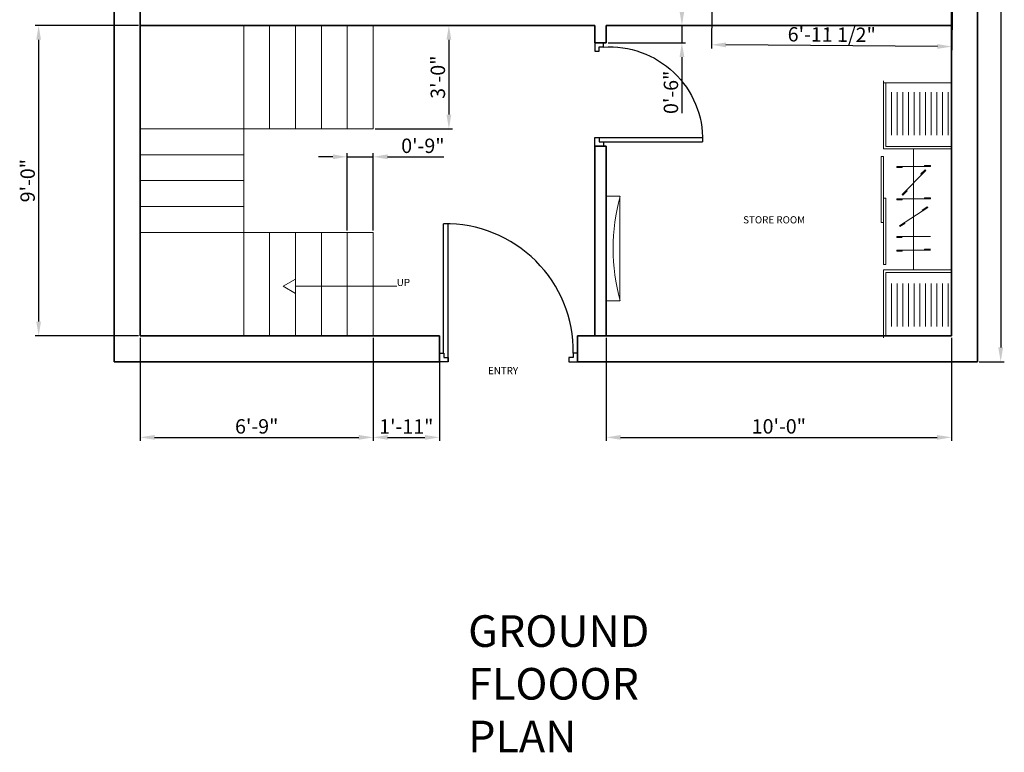
# Model space of a CAD drawing. Units: inches. Extents: x -24887 to 3061, y 1794 to 4919553.
# Tile 4 of 14: x 2132 to 2474, y 1821 to 2076. Entities that reach past the tile are written whole.
import ezdxf

# ---------------------------------------------------------------- set-up
doc = ezdxf.new("R2010")
doc.units = ezdxf.units.IN
for name, color, linetype, lineweight in [('A-ANNO-DIMS', 2, 'Continuous', 18), ('A-AREA-IDEN', 7, 'Continuous', 18), ('A-FLOR-STRS', 4, 'Continuous', 18), ('A-FURN', 8, 'Continuous', 18), ('door', 4, 'Continuous', 25), ('TEXT', 1, 'Continuous', 18), ('TV', 210, 'Continuous', 18), ('wall', 7, 'Continuous', 35)]:
    doc.layers.add(name, color=color, linetype=linetype, lineweight=lineweight)
doc.styles.get("Standard").update_dxf_attribs({"font": 'arial.ttf'})
doc.dimstyles.new('ISO-25', dxfattribs={"dimtxt": 5, "dimasz": 5, "dimexe": 1.25, "dimexo": 0.625, "dimtad": 1, "dimdec": 1, "dimlunit": 3, "dimtxsty": 'Standard', "dimcen": 2.5, "dimadec": 0, "dimazin": 0, "dimtfac": 1, "dimtdec": 1, "dimtmove": 0, "dimatfit": 3, "dimfxl": 1, "dimarcsym": 0})

# ---------------------------------------------------------------- blocks, each defined once
blk = doc.blocks.new('A$C34930FF8')
for p, q in [((600, 1669.3), (600, 2269.3)), ((580, 1690.9), (580, 2252.4)), ((30, 1790.9), (30, 2169.3)), ((80, 1790.9), (80, 2169.3)), ((130, 1790.9), (130, 2169.3)), ((180, 1790.9), (180, 2169.3)), ((230, 1790.9), (230, 2169.3)), ((280, 1790.9), (280, 2169.3)), ((330, 1790.9), (330, 2169.3)), ((380, 1790.9), (380, 2169.3)), ((430, 1790.9), (430, 2169.3)), ((480, 1790.9), (480, 2169.3)), ((530, 1790.9), (530, 2169.3)), ((580, 1690.9), (0, 1690.9)), ((600, 1669.3), (0, 1669.3)), ((335.4, 1666.1), (335.4, 603.1)), ((600, 1603.3), (620, 1603.3)), ((600, 1018.7), (600, 1603.3)), ((620, 1603.3), (620, 1018.7)), ((237.7, 1521.5), (185.4, 1521.5)), ((482.5, 1513), (185.4, 1513)), ((434.8, 1266.1), (227.4, 1478.9)), ((269.7, 1447.7), (233.2, 1485.2)), ((436.7, 1504.4), (482.5, 1504.4)), ((237.7, 1237.7), (185.4, 1237.7)), ((482.5, 1228.2), (185.4, 1228.2)), ((428.7, 1260.1), (392.1, 1297.6)), ((436.7, 1219.7), (482.5, 1219.7)), ((600, 1233.4), (580, 1233.4)), ((580, 1233.4), (580, 648.7)), ((600, 648.7), (600, 1233.4)), ((459.3, 989.3), (209.5, 1150.1)), ((258.1, 1129), (214.1, 1157.3)), ((454.7, 982.1), (410.6, 1010.5)), ((620, 1018.7), (600, 1018.7)), ((482.5, 894.9), (185.4, 894.9)), ((436.7, 886.3), (482.5, 886.3)), ((237.7, 783.9), (185.4, 783.9)), ((482.5, 775.3), (185.4, 775.3)), ((436.7, 766.8), (482.5, 766.8)), ((580, 648.7), (600, 648.7)), ((600, 600), (0, 600)), ((580, 578.3), (0, 578.3)), ((580, 578.3), (580, 16.8)), ((600, 600), (600, 0)), ((30, 478.3), (30, 100)), ((80, 478.3), (80, 100)), ((130, 478.3), (130, 100)), ((180, 478.3), (180, 100)), ((230, 478.3), (230, 100)), ((280, 478.3), (280, 100)), ((330, 478.3), (330, 100)), ((380, 478.3), (380, 100)), ((430, 478.3), (430, 100)), ((480, 478.3), (480, 100)), ((530, 478.3), (530, 100))]:
    blk.add_line(p, q)
at = {"ltscale": 0.05}
for p, q in [((0, 2252.4), (0, 16.8)), ((600, 2252.4), (0, 2252.4)), ((185.4, 1513), (185.4, 1521.5)), ((227.1, 1479.2), (233.2, 1485.2)), ((237.7, 1513), (237.7, 1521.5)), ((436.7, 1513), (436.7, 1504.4)), ((482.5, 1513), (482.5, 1504.4)), ((263.6, 1441.7), (269.7, 1447.7)), ((185.4, 1229.1), (185.4, 1237.7)), ((237.7, 1229.1), (237.7, 1237.7)), ((398.2, 1303.6), (392.1, 1297.6)), ((434.8, 1266.1), (428.7, 1260.1)), ((436.7, 1228.2), (436.7, 1219.7)), ((482.5, 1228.2), (482.5, 1219.7)), ((209.5, 1150.1), (214.1, 1157.3)), ((253.5, 1121.8), (258.1, 1129)), ((415.3, 1017.6), (410.6, 1010.5)), ((459.3, 989.3), (454.7, 982.1)), ((482.5, 894.9), (482.5, 886.3)), ((237.7, 775.3), (237.7, 783.9)), ((436.7, 775.3), (436.7, 766.8)), ((482.5, 775.3), (482.5, 766.8)), ((600, 16.8), (0, 16.8))]:
    blk.add_line(p, q, dxfattribs=at)
blk = doc.blocks.new('*D31')
at = {"layer": 'A-ANNO-DIMS', "color": 0, "lineweight": -2, "transparency": 16777216}
for p, q in [((2465.55, 2316.94), (2474.28, 2316.94)), ((2473.03, 2311.94), (2473.03, 1961.94)), ((2465.55, 1956.94), (2474.28, 1956.94))]:
    blk.add_line(p, q, dxfattribs=at)
at = {"layer": 'A-ANNO-DIMS', "color": 0, "transparency": 16777216}
for points in [[(2472.2, 2311.94), (2473.87, 2311.94), (2473.03, 2316.94)], [(2472.2, 1961.94), (2473.87, 1961.94), (2473.03, 1956.94)]]:
    blk.add_solid(points, dxfattribs=at)
at = {"layer": 'Defpoints', "color": 0, "transparency": 16777216}
for p in [(2464.92, 2316.94), (2464.92, 1956.94), (2473.03, 1956.94)]:
    blk.add_point(p, dxfattribs=at)
at = {"layer": 'A-ANNO-DIMS', "color": 0, "transparency": 16777216, "insert": (2469.85, 2136.94), "char_height": 5, "attachment_point": 5, "rotation": 90}
blk.add_mtext("30'", dxfattribs=at)
blk = doc.blocks.new('DOOR-SINGLE-36IN')
for p, q in [((34.5, 36), (37.5, 36)), ((34.5, 34.5), (34.5, 36)), ((36, 34.5), (34.5, 34.5)), ((36, 33), (36, 34.5)), ((37.5, 36), (37.5, 33)), ((37.5, 33), (36, 33)), ((36, 3), (0, 3)), ((36, 1.5), (0, 1.5)), ((36, 1.5), (34.5, 1.5)), ((34.5, 1.5), (34.5, 0)), ((34.5, 0), (37.5, 0)), ((37.5, 3), (36, 3)), ((36, 3), (36, 1.5)), ((37.5, 0), (37.5, 3))]:
    blk.add_line(p, q)
blk.add_arc((32.32, 2.25), 32.32, 86.1244, 181.3295)
blk = doc.blocks.new('DOOR-ENTRY-48IN')
for p, q in [((1.46, 3), (1.46, 48)), ((3, 0), (3, 48)), ((0, 0), (0, 3)), ((0, 3), (1.5, 3)), ((1.5, 3), (1.5, 1.5)), ((1.5, 1.5), (3, 1.5)), ((3, 1.5), (3, 0)), ((46.5, 1.5), (45, 1.5)), ((45, 1.5), (45, 0)), ((48, 3), (46.5, 3)), ((46.5, 3), (46.5, 1.5)), ((48, 0), (48, 3)), ((3, 0), (0, 0)), ((45, 0), (48, 0))]:
    blk.add_line(p, q)
blk.add_arc((2.23, 3.73), 44.28, 359.0567, 90.9987)
blk = doc.blocks.new('*D61')
at = {"layer": 'A-ANNO-DIMS', "color": 0, "lineweight": -2, "transparency": 16777216}
for p, q in [((2372.6, 2079.98), (2372.49, 2065.97)), ((2456.15, 2079.35), (2456.04, 2065.33)), ((2451.05, 2066.62), (2377.5, 2067.18))]:
    blk.add_line(p, q, dxfattribs=at)
at = {"layer": 'A-ANNO-DIMS', "color": 0, "transparency": 16777216}
for points in [[(2377.51, 2068.01), (2377.49, 2066.34), (2372.5, 2067.22)], [(2451.06, 2067.45), (2451.04, 2065.79), (2456.05, 2066.58)]]:
    blk.add_solid(points, dxfattribs=at)
at = {"layer": 'Defpoints', "color": 0, "transparency": 16777216}
for p in [(2372.6, 2080.61), (2456.15, 2079.98), (2372.5, 2067.22)]:
    blk.add_point(p, dxfattribs=at)
at = {"layer": 'A-ANNO-DIMS', "color": 0, "transparency": 16777216, "insert": (2414.3, 2070.11), "char_height": 5, "attachment_point": 5, "rotation": 359.5659}
blk.add_mtext('6\'-11 1/2"', dxfattribs=at)
blk = doc.blocks.new('*D87')
at = {"layer": 'A-ANNO-DIMS', "color": 0, "lineweight": -2, "transparency": 16777216}
for p, q in [((2335.92, 1965.32), (2335.92, 1929.39)), ((2455.92, 1965.32), (2455.92, 1929.39)), ((2340.92, 1930.64), (2450.92, 1930.64))]:
    blk.add_line(p, q, dxfattribs=at)
at = {"layer": 'A-ANNO-DIMS', "color": 0, "transparency": 16777216}
for points in [[(2340.92, 1931.47), (2340.92, 1929.81), (2335.92, 1930.64)], [(2450.92, 1931.47), (2450.92, 1929.81), (2455.92, 1930.64)]]:
    blk.add_solid(points, dxfattribs=at)
at = {"layer": 'Defpoints', "color": 0, "transparency": 16777216}
for p in [(2335.92, 1965.94), (2455.92, 1965.94), (2455.92, 1930.64)]:
    blk.add_point(p, dxfattribs=at)
at = {"layer": 'A-ANNO-DIMS', "color": 0, "transparency": 16777216, "insert": (2395.92, 1933.82), "char_height": 5, "attachment_point": 5}
blk.add_mtext('10\'-0"', dxfattribs=at)
blk = doc.blocks.new('*D90')
at = {"layer": 'A-ANNO-DIMS', "color": 0, "lineweight": -2, "transparency": 16777216}
for p, q in [((2173.3, 2073.94), (2137.37, 2073.94)), ((2138.62, 2068.94), (2138.62, 1970.94)), ((2173.3, 1965.94), (2137.37, 1965.94))]:
    blk.add_line(p, q, dxfattribs=at)
at = {"layer": 'A-ANNO-DIMS', "color": 0, "transparency": 16777216}
for points in [[(2137.79, 2068.94), (2139.46, 2068.94), (2138.62, 2073.94)], [(2137.79, 1970.94), (2139.46, 1970.94), (2138.62, 1965.94)]]:
    blk.add_solid(points, dxfattribs=at)
at = {"layer": 'Defpoints', "color": 0, "transparency": 16777216}
for p in [(2173.92, 2073.94), (2138.62, 1965.94), (2173.92, 1965.94)]:
    blk.add_point(p, dxfattribs=at)
at = {"layer": 'A-ANNO-DIMS', "color": 0, "transparency": 16777216, "insert": (2135.45, 2019.94), "char_height": 5, "attachment_point": 5, "rotation": 90}
blk.add_mtext('9\'-0"', dxfattribs=at)
blk = doc.blocks.new('*D93')
at = {"layer": 'A-ANNO-DIMS', "color": 0, "lineweight": -2, "transparency": 16777216}
for p, q in [((2173.92, 1965.32), (2173.92, 1929.39)), ((2254.92, 1965.32), (2254.92, 1929.39)), ((2178.92, 1930.64), (2249.92, 1930.64))]:
    blk.add_line(p, q, dxfattribs=at)
at = {"layer": 'A-ANNO-DIMS', "color": 0, "transparency": 16777216}
for points in [[(2178.92, 1931.47), (2178.92, 1929.81), (2173.92, 1930.64)], [(2249.92, 1931.47), (2249.92, 1929.81), (2254.92, 1930.64)]]:
    blk.add_solid(points, dxfattribs=at)
at = {"layer": 'Defpoints', "color": 0, "transparency": 16777216}
for p in [(2173.92, 1965.94), (2254.92, 1965.94), (2254.92, 1930.64)]:
    blk.add_point(p, dxfattribs=at)
at = {"layer": 'A-ANNO-DIMS', "color": 0, "transparency": 16777216, "insert": (2214.42, 1933.82), "char_height": 5, "attachment_point": 5}
blk.add_mtext('6\'-9"', dxfattribs=at)
blk = doc.blocks.new('*D94')
at = {"layer": 'A-ANNO-DIMS', "color": 0, "lineweight": -2, "transparency": 16777216}
for p, q in [((2254.92, 1965.32), (2254.92, 1929.39)), ((2277.92, 1965.32), (2277.92, 1929.39)), ((2259.92, 1930.64), (2272.92, 1930.64))]:
    blk.add_line(p, q, dxfattribs=at)
at = {"layer": 'A-ANNO-DIMS', "color": 0, "transparency": 16777216}
for points in [[(2259.92, 1931.47), (2259.92, 1929.81), (2254.92, 1930.64)], [(2272.92, 1931.47), (2272.92, 1929.81), (2277.92, 1930.64)]]:
    blk.add_solid(points, dxfattribs=at)
at = {"layer": 'Defpoints', "color": 0, "transparency": 16777216}
for p in [(2254.92, 1965.94), (2277.92, 1965.94), (2277.92, 1930.64)]:
    blk.add_point(p, dxfattribs=at)
at = {"layer": 'A-ANNO-DIMS', "color": 0, "transparency": 16777216, "insert": (2266.42, 1933.78), "char_height": 5, "attachment_point": 5}
blk.add_mtext('1\'-11"', dxfattribs=at)
blk = doc.blocks.new('*D95')
at = {"layer": 'A-ANNO-DIMS', "color": 0, "lineweight": -2, "transparency": 16777216}
for p, q in [((2240.92, 2028.24), (2235.92, 2028.24)), ((2245.92, 2002.57), (2245.92, 2029.49)), ((2245.92, 2028.24), (2254.92, 2028.24)), ((2254.92, 2002.57), (2254.92, 2029.49)), ((2259.92, 2028.24), (2279.46, 2028.24))]:
    blk.add_line(p, q, dxfattribs=at)
at = {"layer": 'A-ANNO-DIMS', "color": 0, "transparency": 16777216}
for points in [[(2240.92, 2029.07), (2240.92, 2027.41), (2245.92, 2028.24)], [(2259.92, 2029.07), (2259.92, 2027.41), (2254.92, 2028.24)]]:
    blk.add_solid(points, dxfattribs=at)
at = {"layer": 'Defpoints', "color": 0, "transparency": 16777216}
for p in [(2254.92, 2028.24), (2245.92, 2001.94), (2254.92, 2001.94)]:
    blk.add_point(p, dxfattribs=at)
at = {"layer": 'A-ANNO-DIMS', "color": 0, "transparency": 16777216, "insert": (2272.19, 2031.42), "char_height": 5, "attachment_point": 5}
blk.add_mtext('0\'-9"', dxfattribs=at)
blk = doc.blocks.new('*D96')
at = {"layer": 'A-ANNO-DIMS', "color": 0, "lineweight": -2, "transparency": 16777216}
for p, q in [((2255.55, 2073.94), (2282.47, 2073.94)), ((2281.22, 2068.94), (2281.22, 2042.94)), ((2255.55, 2037.94), (2282.47, 2037.94))]:
    blk.add_line(p, q, dxfattribs=at)
at = {"layer": 'A-ANNO-DIMS', "color": 0, "transparency": 16777216}
for points in [[(2280.39, 2068.94), (2282.06, 2068.94), (2281.22, 2073.94)], [(2280.39, 2042.94), (2282.06, 2042.94), (2281.22, 2037.94)]]:
    blk.add_solid(points, dxfattribs=at)
at = {"layer": 'Defpoints', "color": 0, "transparency": 16777216}
for p in [(2254.92, 2073.94), (2254.92, 2037.94), (2281.22, 2037.94)]:
    blk.add_point(p, dxfattribs=at)
at = {"layer": 'A-ANNO-DIMS', "color": 0, "transparency": 16777216, "insert": (2278.04, 2055.94), "char_height": 5, "attachment_point": 5, "rotation": 90}
blk.add_mtext('3\'-0"', dxfattribs=at)
blk = doc.blocks.new('*D98')
at = {"layer": 'A-ANNO-DIMS', "color": 0, "lineweight": -2, "transparency": 16777216}
for p, q in [((2362.22, 2078.94), (2362.22, 2083.94)), ((2336.55, 2073.94), (2363.47, 2073.94)), ((2362.22, 2073.94), (2362.22, 2067.94)), ((2336.55, 2067.94), (2363.47, 2067.94)), ((2362.22, 2062.94), (2362.22, 2043.4))]:
    blk.add_line(p, q, dxfattribs=at)
at = {"layer": 'A-ANNO-DIMS', "color": 0, "transparency": 16777216}
for points in [[(2361.39, 2078.94), (2363.06, 2078.94), (2362.22, 2073.94)], [(2361.39, 2062.94), (2363.06, 2062.94), (2362.22, 2067.94)]]:
    blk.add_solid(points, dxfattribs=at)
at = {"layer": 'Defpoints', "color": 0, "transparency": 16777216}
for p in [(2335.92, 2073.94), (2335.92, 2067.94), (2362.22, 2067.94)]:
    blk.add_point(p, dxfattribs=at)
at = {"layer": 'A-ANNO-DIMS', "color": 0, "transparency": 16777216, "insert": (2359.05, 2050.67), "char_height": 5, "attachment_point": 5, "rotation": 90}
blk.add_mtext('0\'-6"', dxfattribs=at)

msp = doc.modelspace()

# ---------------------------------------------------------------- linework, layer by layer
at = {"layer": 'A-FLOR-STRS'}
for p, q in [((2209.92, 2073.94), (2173.92, 2073.94)), ((2173.92, 2073.94), (2173.92, 2037.94)), ((2209.92, 2037.94), (2209.92, 2073.94)), ((2209.92, 2073.94), (2254.92, 2073.94)), ((2218.92, 2037.94), (2218.92, 2073.94)), ((2227.92, 2037.94), (2227.92, 2073.94)), ((2236.92, 2037.94), (2236.92, 2073.94)), ((2245.92, 2037.94), (2245.92, 2073.94)), ((2254.92, 2037.94), (2254.92, 2073.94)), ((2173.92, 2037.94), (2209.92, 2037.94)), ((2173.92, 2037.94), (2173.92, 2001.94)), ((2209.92, 2037.94), (2209.92, 2001.94)), ((2209.92, 2037.94), (2254.92, 2037.94)), ((2173.92, 2028.94), (2209.92, 2028.94)), ((2173.92, 2019.94), (2209.92, 2019.94)), ((2173.92, 2010.94), (2209.92, 2010.94)), ((2209.92, 2001.94), (2173.92, 2001.94)), ((2173.92, 2001.94), (2173.92, 1965.94)), ((2173.92, 2001.94), (2209.92, 2001.94)), ((2209.92, 1965.94), (2209.92, 2001.94)), ((2209.92, 1965.94), (2209.92, 2001.94)), ((2209.92, 2001.94), (2254.92, 2001.94)), ((2218.92, 1965.94), (2218.92, 2001.94)), ((2227.92, 1965.94), (2227.92, 2001.94)), ((2236.92, 1965.94), (2236.92, 2001.94)), ((2245.92, 1965.94), (2245.92, 2001.94)), ((2254.92, 1965.94), (2254.92, 2001.94)), ((2263.1, 1983.21), (2227.92, 1983.21)), ((2173.92, 1965.94), (2209.92, 1965.94)), ((2209.92, 1965.94), (2254.92, 1965.94))]:
    msp.add_line(p, q, dxfattribs=at)
msp.add_lwpolyline([(2227.92, 1980.69), (2227.92, 1985.72), (2223.57, 1983.21)], close=True, dxfattribs=at)
at = {"layer": 'TV'}
msp.add_lwpolyline([(2335.92, 2014.51), (2340.7, 2014.51), (2340.7, 1978.17), (2335.92, 1978.17)], close=True, dxfattribs=at)
msp.add_arc((2408.64, 1996.34), 70.32, 165.0255, 194.9745, dxfattribs=at)
at = {"layer": 'wall'}
for p, q in [((2164.92, 2316.94), (2164.92, 1956.94)), ((2464.92, 1956.94), (2464.92, 2316.94)), ((2173.92, 2307.94), (2173.92, 1965.94)), ((2455.92, 1965.94), (2455.92, 2307.94)), ((2331.92, 2073.94), (2173.92, 2073.94)), ((2331.92, 2067.94), (2331.92, 2073.94)), ((2455.92, 2073.94), (2335.92, 2073.94)), ((2335.92, 2067.94), (2335.92, 2073.94)), ((2335.92, 2067.94), (2331.92, 2067.94)), ((2331.92, 1965.94), (2331.92, 2031.94)), ((2335.92, 2031.94), (2331.92, 2031.94)), ((2335.92, 1965.94), (2335.92, 2031.94)), ((2173.92, 1965.94), (2277.92, 1965.94)), ((2277.92, 1965.94), (2277.92, 1956.94)), ((2325.92, 1965.94), (2325.92, 1956.94)), ((2325.92, 1965.94), (2455.92, 1965.94)), ((2164.92, 1956.94), (2277.92, 1956.94)), ((2325.92, 1956.94), (2464.92, 1956.94))]:
    msp.add_line(p, q, dxfattribs=at)

# ---------------------------------------------------------------- block references
at = {"layer": 'A-FURN', "xscale": -0.0393700787401575, "yscale": 0.0393700787401575, "zscale": 0.0393700787401575}
msp.add_blockref('A$C34930FF8', (2455.92, 1965.28), dxfattribs=at)
at = {"layer": 'door', "extrusion": (0, 0, -1), "zscale": -1}
msp.add_blockref('DOOR-SINGLE-36IN', (-2369.42, 2031.94), dxfattribs=at)
at = {"layer": 'door'}
msp.add_blockref('DOOR-ENTRY-48IN', (2277.92, 1956.94), dxfattribs=at)

# ---------------------------------------------------------------- texts
at = {"layer": 'A-AREA-IDEN', "insert": (2383.51, 2007.57), "char_height": 2.5, "attachment_point": 1}
msp.add_mtext_dynamic_manual_height_columns('STORE ROOM', width=34.2323, gutter_width=12.5, heights=[0], dxfattribs=at)
at = {"layer": 'TEXT', "attachment_point": 1}
for s, insert, char_height in [('UP', (2263.1, 1985.79), 2.5), ('ENTRY', (2294.81, 1955.1), 2.5), ('GROUND\\PFLOOOR\\PPLAN', (2287.92, 1868.76), 11)]:
    msp.add_mtext_dynamic_manual_height_columns(s, width=34.2323, gutter_width=12.5, heights=[0], dxfattribs=dict(at, insert=insert, char_height=char_height))

# ---------------------------------------------------------------- dimensions: what is measured, and where the dimension line sits
at = {"layer": 'A-ANNO-DIMS'}
for base, p1, p2, angle, override, picture, middle in [((2473.03, 1956.94), (2464.92, 2316.94), (2464.92, 1956.94), 90, {"dimclrd": 0, "dimclre": 0, "dimclrt": 0}, '*D31', (2469.85, 2136.94)), ((2362.22, 2067.94), (2335.92, 2073.94), (2335.92, 2067.94), 270, {"dimdec": 1, "dimlfac": 1, "dimrnd": 0, "dimzin": 1, "dimdsep": 46, "dimlunit": 4, "dimfrac": 2}, '*D98', (2359.05, 2050.67)), ((2372.5, 2067.22), (2456.15, 2079.98), (2372.6, 2080.61), 179.5659, {"dimdec": 1, "dimlfac": 1, "dimrnd": 0, "dimzin": 1, "dimdsep": 46, "dimlunit": 4, "dimfrac": 2}, '*D61', (2414.3, 2070.11)), ((2138.62, 1965.94), (2173.92, 2073.94), (2173.92, 1965.94), 90, {"dimdec": 1, "dimlfac": 1, "dimrnd": 0, "dimzin": 1, "dimdsep": 46, "dimlunit": 4, "dimfrac": 2}, '*D90', (2135.45, 2019.94)), ((2281.22, 2037.94), (2254.92, 2073.94), (2254.92, 2037.94), 270, {"dimdec": 1, "dimlfac": 1, "dimrnd": 0, "dimzin": 1, "dimdsep": 46, "dimlunit": 4, "dimfrac": 2}, '*D96', (2278.04, 2055.94))]:
    dim = msp.add_linear_dim(base=base, p1=p1, p2=p2, angle=angle, dimstyle='ISO-25', override=override, dxfattribs=at)
    dim.commit()
    dim.dimension.update_dxf_attribs({"geometry": picture, "text_midpoint": middle})
for base, p1, p2, picture, middle in [((2254.92, 2028.24), (2245.92, 2001.94), (2254.92, 2001.94), '*D95', (2272.19, 2031.42)), ((2254.92, 1930.64), (2173.92, 1965.94), (2254.92, 1965.94), '*D93', (2214.42, 1933.82)), ((2277.92, 1930.64), (2254.92, 1965.94), (2277.92, 1965.94), '*D94', (2266.42, 1933.78)), ((2455.92, 1930.64), (2335.92, 1965.94), (2455.92, 1965.94), '*D87', (2395.92, 1933.82))]:
    dim = msp.add_linear_dim(base=base, p1=p1, p2=p2, dimstyle='ISO-25', override={"dimdec": 1, "dimlfac": 1, "dimrnd": 0, "dimzin": 1, "dimdsep": 46, "dimlunit": 4, "dimfrac": 2}, dxfattribs=at)
    dim.commit()
    dim.dimension.update_dxf_attribs({"geometry": picture, "text_midpoint": middle})

doc.saveas('drawing.dxf')
